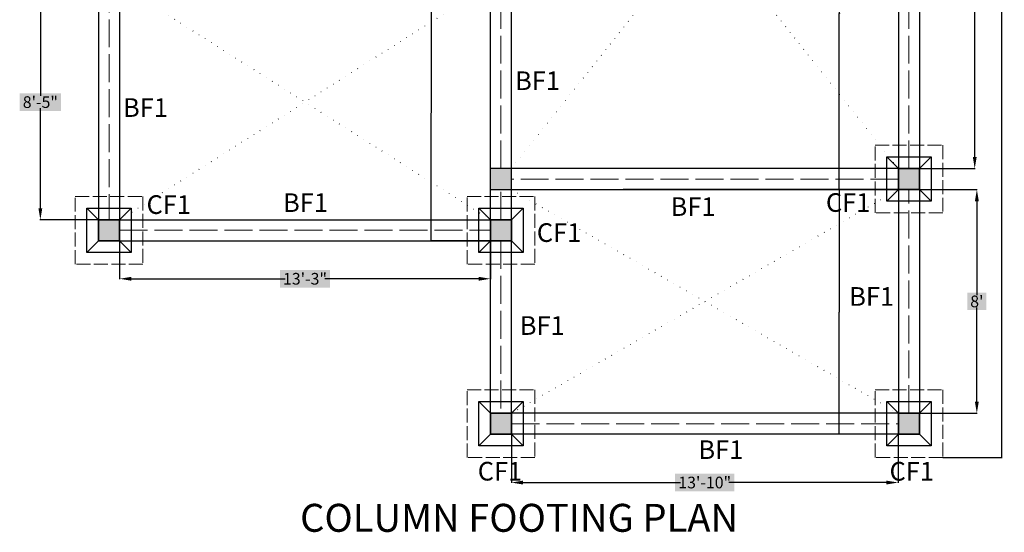
# Model space of a CAD drawing. Units: inches. Extents: x -35 to 832, y -515 to 219.
# Tile 6 of 7: x 410 to 832, y -295 to -75. Entities that reach past the tile are written whole.
import ezdxf

# ---------------------------------------------------------------- set-up
doc = ezdxf.new("R2010")
doc.units = ezdxf.units.IN
doc.header["$MEASUREMENT"] = 0
doc.linetypes.add('ACAD_ISO02W100', pattern=[15, 12, -3])
doc.linetypes.add('ACAD_ISO07W100', pattern=[3, 0, -3])
for name, color, linetype, lineweight in [('G-ANNO-TEXT', 7, 'Continuous', 35), ('S-ANNO-DIMS', 2, 'Continuous', 18), ('S-ANNO-TEXT', 7, 'Continuous', 18), ('S-BEAM', 6, 'Continuous', 25), ('S-BEAM-CNTR', 2, 'ACAD_ISO02W100', 13), ('S-COLS', 4, 'Continuous', 35), ('S-COLS-PATT', 8, 'Continuous', 13), ('S-FNDN', 4, 'Continuous', 25), ('S-FNDN-HIDN', 7, 'ACAD_ISO02W100', 18), ('S-FNDN-REFR', 8, 'ACAD_ISO07W100', 13)]:
    doc.layers.add(name, color=color, linetype=linetype, lineweight=lineweight)
doc.styles.get("Standard").update_dxf_attribs({"font": 'arial.ttf'})
doc.dimstyles.get("Standard").update_dxf_attribs({"dimtxt": 0.18, "dimasz": 0.18, "dimexe": 0.18, "dimexo": 0.0625, "dimgap": 0.09, "dimtad": 0, "dimtih": 1, "dimtoh": 1, "dimdec": 1, "dimzin": 0, "dimdsep": 46, "dimlunit": 4, "dimtxsty": 'Standard', "dimcen": 0.09, "dimclrd": 211, "dimclre": 4, "dimclrt": 3, "dimadec": 0, "dimazin": 0, "dimtfac": 0.5, "dimtdec": 1, "dimtofl": 0, "dimtmove": 0, "dimatfit": 3, "dimfxl": 1, "dimtfill": 2, "dimtfillclr": 61, "dimtolj": 1, "dimtzin": 0, "dimarcsym": 0})

# ---------------------------------------------------------------- blocks, each defined once
blk = doc.blocks.new('*D28')
at = {"layer": 'Defpoints', "color": 0, "transparency": 16777216}
for p in [(620.57, -248.58), (786.4, -248.58), (786.4, -273.78)]:
    blk.add_point(p, dxfattribs=at)
at = {"layer": 'S-ANNO-DIMS', "color": 0, "lineweight": -2, "transparency": 16777216}
for p, q in [((620.57, -248.64), (620.57, -273.96)), ((786.4, -248.64), (786.4, -273.96)), ((625.57, -273.78), (693.1, -273.78)), ((781.4, -273.78), (713.87, -273.78))]:
    blk.add_line(p, q, dxfattribs=at)
at = {"layer": 'S-ANNO-DIMS', "color": 0, "transparency": 16777216}
for points in [[(625.57, -272.95), (625.57, -274.62), (620.57, -273.78)], [(781.4, -272.95), (781.4, -274.62), (786.4, -273.78)]]:
    blk.add_solid(points, dxfattribs=at)
at = {"layer": 'S-ANNO-DIMS', "color": 0, "transparency": 16777216, "insert": (703.49, -273.78), "char_height": 5, "attachment_point": 5, "bg_fill": 1, "box_fill_scale": 1.25, "bg_fill_color": 61, "bg_fill_transparency": 0}
blk.add_mtext('\\A1;13\'-10"', dxfattribs=at)
blk = doc.blocks.new('*D29')
at = {"layer": 'Defpoints', "color": 0, "transparency": 16777216}
for p in [(452.57, -165.58), (611.57, -165.58), (611.57, -186.37)]:
    blk.add_point(p, dxfattribs=at)
at = {"layer": 'S-ANNO-DIMS', "color": 0, "lineweight": -2, "transparency": 16777216}
for p, q in [((452.57, -165.64), (452.57, -186.55)), ((611.57, -165.64), (611.57, -186.55)), ((457.57, -186.37), (523.63, -186.37)), ((606.57, -186.37), (540.51, -186.37))]:
    blk.add_line(p, q, dxfattribs=at)
at = {"layer": 'S-ANNO-DIMS', "color": 0, "transparency": 16777216}
for points in [[(457.57, -185.54), (457.57, -187.21), (452.57, -186.37)], [(606.57, -185.54), (606.57, -187.21), (611.57, -186.37)]]:
    blk.add_solid(points, dxfattribs=at)
at = {"layer": 'S-ANNO-DIMS', "color": 0, "transparency": 16777216, "insert": (532.07, -186.37), "char_height": 5, "attachment_point": 5, "bg_fill": 1, "box_fill_scale": 1.25, "bg_fill_color": 61, "bg_fill_transparency": 0}
blk.add_mtext('\\A1;13\'-3"', dxfattribs=at)
blk = doc.blocks.new('*D30')
at = {"layer": 'Defpoints', "color": 0, "transparency": 16777216}
for p in [(786.57, -148.08), (786.57, -244.08), (820.2, -244.08)]:
    blk.add_point(p, dxfattribs=at)
at = {"layer": 'S-ANNO-DIMS', "color": 0, "lineweight": -2, "transparency": 16777216}
for p, q in [((786.63, -148.08), (820.38, -148.08)), ((820.2, -153.08), (820.2, -193.43)), ((820.2, -239.08), (820.2, -198.72)), ((786.63, -244.08), (820.38, -244.08))]:
    blk.add_line(p, q, dxfattribs=at)
at = {"layer": 'S-ANNO-DIMS', "color": 0, "transparency": 16777216}
for points in [[(819.37, -153.08), (821.03, -153.08), (820.2, -148.08)], [(819.37, -239.08), (821.03, -239.08), (820.2, -244.08)]]:
    blk.add_solid(points, dxfattribs=at)
at = {"layer": 'S-ANNO-DIMS', "color": 0, "transparency": 16777216, "insert": (820.2, -196.08), "char_height": 5, "attachment_point": 5, "bg_fill": 1, "box_fill_scale": 1.25, "bg_fill_color": 61, "bg_fill_transparency": 0}
blk.add_mtext("\\A1;8'", dxfattribs=at)
blk = doc.blocks.new('*D31')
at = {"layer": 'Defpoints', "color": 0, "transparency": 16777216}
for p in [(786.57, 2.92), (819.29, 2.92), (786.57, -139.08)]:
    blk.add_point(p, dxfattribs=at)
at = {"layer": 'S-ANNO-DIMS', "color": 0, "lineweight": -2, "transparency": 16777216}
for p, q in [((786.63, 2.92), (819.47, 2.92)), ((819.29, -2.08), (819.29, -65.43)), ((819.29, -134.08), (819.29, -70.72)), ((786.63, -139.08), (819.47, -139.08))]:
    blk.add_line(p, q, dxfattribs=at)
at = {"layer": 'S-ANNO-DIMS', "color": 0, "transparency": 16777216}
for points in [[(818.46, -2.08), (820.13, -2.08), (819.29, 2.92)], [(818.46, -134.08), (820.13, -134.08), (819.29, -139.08)]]:
    blk.add_solid(points, dxfattribs=at)
at = {"layer": 'S-ANNO-DIMS', "color": 0, "transparency": 16777216, "insert": (819.29, -68.08), "char_height": 5, "attachment_point": 5, "bg_fill": 1, "box_fill_scale": 1.25, "bg_fill_color": 61, "bg_fill_transparency": 0}
blk.add_mtext('\\A1;11\'-10"', dxfattribs=at)
blk = doc.blocks.new('*D38')
at = {"layer": 'Defpoints', "color": 0, "transparency": 16777216}
for p in [(448.07, -60.08), (418.57, -161.08), (448.07, -161.08)]:
    blk.add_point(p, dxfattribs=at)
at = {"layer": 'S-ANNO-DIMS', "color": 0, "lineweight": -2, "transparency": 16777216}
for p, q in [((448.01, -60.08), (418.39, -60.08)), ((418.57, -65.08), (418.57, -107.93)), ((418.57, -156.08), (418.57, -113.22)), ((448.01, -161.08), (418.39, -161.08))]:
    blk.add_line(p, q, dxfattribs=at)
at = {"layer": 'S-ANNO-DIMS', "color": 0, "transparency": 16777216}
for points in [[(417.74, -65.08), (419.41, -65.08), (418.57, -60.08)], [(417.74, -156.08), (419.41, -156.08), (418.57, -161.08)]]:
    blk.add_solid(points, dxfattribs=at)
at = {"layer": 'S-ANNO-DIMS', "color": 0, "transparency": 16777216, "insert": (418.57, -110.58), "char_height": 5, "attachment_point": 5, "bg_fill": 1, "box_fill_scale": 1.25, "bg_fill_color": 61, "bg_fill_transparency": 0}
blk.add_mtext('\\A1;8\'-5"', dxfattribs=at)
blk = doc.blocks.new('CF1-TAPERED-FOOTING')
for p, q in [((0, 19), (19, 19)), ((0, 0), (0, 19)), ((0, 19), (5, 14)), ((14, 14), (19, 19)), ((19, 19), (19, 0)), ((0, 0), (5, 5)), ((14, 5), (19, 0)), ((19, 0), (0, 0))]:
    blk.add_line(p, q)
blk = doc.blocks.new('CF1-FOOTING-LIMIT')
at = {"ltscale": 0.5}
for p, q in [((0, 29), (29, 29)), ((0, 0), (0, 29)), ((29, 29), (29, 0)), ((29, 0), (0, 0))]:
    blk.add_line(p, q, dxfattribs=at)
blk = doc.blocks.new('*D140')
at = {"layer": 'Defpoints', "color": 0, "transparency": 16777216}
for p in [(805.57, 193.92), (805.57, -263.08), (830.92, -263.08)]:
    blk.add_point(p, dxfattribs=at)
at = {"layer": 'S-ANNO-DIMS', "color": 4, "lineweight": -2, "transparency": 16777216}
for p, q in [((805.63, 193.92), (831.1, 193.92)), ((805.63, -263.08), (831.1, -263.08))]:
    blk.add_line(p, q, dxfattribs=at)
at = {"layer": 'S-ANNO-DIMS', "color": 211, "lineweight": -2, "transparency": 16777216}
for p, q in [((830.92, 193.74), (830.92, -34.39)), ((830.92, -262.9), (830.92, -34.76))]:
    blk.add_line(p, q, dxfattribs=at)
at = {"layer": 'S-ANNO-DIMS', "color": 211, "transparency": 16777216}
for points in [[(830.89, 193.74), (830.95, 193.74), (830.92, 193.92)], [(830.89, -262.9), (830.95, -262.9), (830.92, -263.08)]]:
    blk.add_solid(points, dxfattribs=at)
at = {"layer": 'S-ANNO-DIMS', "color": 3, "transparency": 16777216, "insert": (830.92, -34.58), "char_height": 0.18, "attachment_point": 5, "bg_fill": 1, "box_fill_scale": 1.25, "bg_fill_color": 61, "bg_fill_transparency": 0}
blk.add_mtext('\\A1;38\'-1"', dxfattribs=at)
blk = doc.blocks.new('*D145')
at = {"layer": 'Defpoints', "color": 0, "transparency": 16777216}
for p in [(586.22, -60.08), (611.57, -60.08), (611.57, -170.08)]:
    blk.add_point(p, dxfattribs=at)
at = {"layer": 'S-ANNO-DIMS', "color": 4, "lineweight": -2, "transparency": 16777216}
for p, q in [((611.51, -60.08), (586.04, -60.08)), ((611.51, -170.08), (586.04, -170.08))]:
    blk.add_line(p, q, dxfattribs=at)
at = {"layer": 'S-ANNO-DIMS', "color": 211, "lineweight": -2, "transparency": 16777216}
for p, q in [((586.22, -60.26), (586.22, -114.89)), ((586.22, -169.9), (586.22, -115.26))]:
    blk.add_line(p, q, dxfattribs=at)
at = {"layer": 'S-ANNO-DIMS', "color": 211, "transparency": 16777216}
for points in [[(586.19, -60.26), (586.25, -60.26), (586.22, -60.08)], [(586.19, -169.9), (586.25, -169.9), (586.22, -170.08)]]:
    blk.add_solid(points, dxfattribs=at)
at = {"layer": 'S-ANNO-DIMS', "color": 3, "transparency": 16777216, "insert": (586.22, -115.08), "char_height": 0.18, "attachment_point": 5, "bg_fill": 1, "box_fill_scale": 1.25, "bg_fill_color": 61, "bg_fill_transparency": 0}
blk.add_mtext('\\A1;9\'-2"', dxfattribs=at)
blk = doc.blocks.new('*D148')
at = {"layer": 'Defpoints', "color": 0, "transparency": 16777216}
for p in [(761.22, 2.92), (786.57, 2.92), (786.57, -148.08)]:
    blk.add_point(p, dxfattribs=at)
at = {"layer": 'S-ANNO-DIMS', "color": 4, "lineweight": -2, "transparency": 16777216}
for p, q in [((786.51, 2.92), (761.04, 2.92)), ((786.51, -148.08), (761.04, -148.08))]:
    blk.add_line(p, q, dxfattribs=at)
at = {"layer": 'S-ANNO-DIMS', "color": 211, "lineweight": -2, "transparency": 16777216}
for p, q in [((761.22, 2.74), (761.22, -72.39)), ((761.22, -147.9), (761.22, -72.76))]:
    blk.add_line(p, q, dxfattribs=at)
at = {"layer": 'S-ANNO-DIMS', "color": 211, "transparency": 16777216}
for points in [[(761.19, 2.74), (761.25, 2.74), (761.22, 2.92)], [(761.19, -147.9), (761.25, -147.9), (761.22, -148.08)]]:
    blk.add_solid(points, dxfattribs=at)
at = {"layer": 'S-ANNO-DIMS', "color": 3, "transparency": 16777216, "insert": (761.22, -72.58), "char_height": 0.18, "attachment_point": 5, "bg_fill": 1, "box_fill_scale": 1.25, "bg_fill_color": 61, "bg_fill_transparency": 0}
blk.add_mtext('\\A1;12\'-7"', dxfattribs=at)
blk = doc.blocks.new('*D149')
at = {"layer": 'Defpoints', "color": 0, "transparency": 16777216}
for p in [(761.22, -148.08), (786.57, -148.08), (786.57, -253.08)]:
    blk.add_point(p, dxfattribs=at)
at = {"layer": 'S-ANNO-DIMS', "color": 4, "lineweight": -2, "transparency": 16777216}
for p, q in [((786.51, -148.08), (761.04, -148.08)), ((786.51, -253.08), (761.04, -253.08))]:
    blk.add_line(p, q, dxfattribs=at)
at = {"layer": 'S-ANNO-DIMS', "color": 211, "lineweight": -2, "transparency": 16777216}
for p, q in [((761.22, -148.26), (761.22, -200.39)), ((761.22, -252.9), (761.22, -200.76))]:
    blk.add_line(p, q, dxfattribs=at)
at = {"layer": 'S-ANNO-DIMS', "color": 211, "transparency": 16777216}
for points in [[(761.19, -148.26), (761.25, -148.26), (761.22, -148.08)], [(761.19, -252.9), (761.25, -252.9), (761.22, -253.08)]]:
    blk.add_solid(points, dxfattribs=at)
at = {"layer": 'S-ANNO-DIMS', "color": 3, "transparency": 16777216, "insert": (761.22, -200.58), "char_height": 0.18, "attachment_point": 5, "bg_fill": 1, "box_fill_scale": 1.25, "bg_fill_color": 61, "bg_fill_transparency": 0}
blk.add_mtext('\\A1;8\'-9"', dxfattribs=at)

msp = doc.modelspace()

# ---------------------------------------------------------------- hatches: boundary and pattern name
at = {"layer": 'S-COLS-PATT'}
h = msp.add_hatch(color=256, dxfattribs=at)
h.dxf.hatch_style = 1
h.paths.add_polyline_path([(443.57, 183.92), (443.57, 174.92), (452.57, 174.92), (452.57, 183.92)])
h.paths.add_polyline_path([(620.57, 183.92), (611.57, 183.92), (611.57, 174.92), (620.57, 174.92)])
h.paths.add_polyline_path([(786.57, 183.92), (786.57, 174.92), (795.57, 174.92), (795.57, 183.92)])
h.paths.add_polyline_path([(620.57, 78.92), (611.57, 78.92), (611.57, 69.92), (620.57, 69.92)])
h.paths.add_polyline_path([(659.57, 78.92), (659.57, 69.92), (668.57, 69.92), (668.57, 78.92)])
h.paths.add_polyline_path([(795.57, 78.92), (786.57, 78.92), (786.57, 69.92), (795.57, 69.92)])
h.paths.add_polyline_path([(668.57, 11.92), (659.57, 11.92), (659.57, 2.92), (668.57, 2.92)])
h.paths.add_polyline_path([(795.57, 11.92), (786.57, 11.92), (786.57, 2.92), (795.57, 2.92)])
h.paths.add_polyline_path([(611.57, 17.92), (611.57, 8.92), (620.57, 8.92), (620.57, 17.92)])
h.paths.add_polyline_path([(557.57, 17.92), (548.57, 17.92), (548.57, 8.92), (557.57, 8.92)])
h.paths.add_polyline_path([(443.57, 8.92), (452.57, 8.92), (452.57, 17.92), (443.57, 17.92)])
h.paths.add_polyline_path([(443.57, -51.08), (443.57, -60.08), (452.57, -60.08), (452.57, -51.08)])
h.paths.add_polyline_path([(557.57, -51.08), (548.57, -51.08), (548.57, -60.08), (557.57, -60.08)])
h.paths.add_polyline_path([(620.57, -60.08), (620.57, -51.08), (611.57, -51.08), (611.57, -60.08)])
h.paths.add_polyline_path([(620.57, -139.08), (611.57, -139.08), (611.57, -148.08), (620.57, -148.08)])
h.paths.add_polyline_path([(786.57, -148.08), (795.57, -148.08), (795.57, -139.08), (786.57, -139.08)])
h.paths.add_polyline_path([(443.57, -161.08), (443.57, -170.08), (452.57, -170.08), (452.57, -161.08)])
h.paths.add_polyline_path([(611.57, -161.08), (611.57, -170.08), (620.57, -170.08), (620.57, -161.08)])
h.paths.add_polyline_path([(620.57, -244.08), (611.57, -244.08), (611.57, -253.08), (620.57, -253.08)])
h.paths.add_polyline_path([(786.57, -244.08), (786.57, -253.08), (795.57, -253.08), (795.57, -244.08)])

# ---------------------------------------------------------------- linework, layer by layer
at = {"layer": 'S-BEAM'}
for p, q in [((611.57, -142.58), (611.57, 78.92)), ((620.57, -142.58), (620.57, 69.92)), ((795.57, 11.92), (795.57, -139.08)), ((786.57, 2.92), (786.57, -139.08)), ((443.57, -51.08), (443.57, -170.08)), ((452.57, -60.08), (452.57, -161.08)), ((795.57, -60.08), (795.57, -253.08)), ((786.57, -139.08), (611.57, -139.08)), ((611.57, -253.08), (611.57, -139.08)), ((620.57, -244.08), (620.57, -139.08)), ((611.57, -148.08), (786.57, -148.08)), ((786.57, -148.08), (668.57, -148.08)), ((786.57, -148.08), (786.57, -244.08)), ((452.57, -161.08), (620.57, -161.08)), ((443.57, -170.08), (611.57, -170.08)), ((786.57, -244.08), (620.57, -244.08)), ((795.57, -253.08), (611.57, -253.08))]:
    msp.add_line(p, q, dxfattribs=at)
at = {"layer": 'S-BEAM-CNTR'}
for p, q in [((616.07, -139.08), (616.07, 74.42)), ((791.07, -139.08), (791.07, 2.92)), ((448.07, -60.08), (448.07, -161.08)), ((786.57, -143.58), (620.57, -143.58)), ((616.07, -161.08), (616.07, -148.08)), ((791.07, -244.08), (791.07, -148.08)), ((452.57, -165.58), (611.57, -165.58)), ((616.07, -170.08), (616.07, -244.08)), ((620.57, -248.58), (786.57, -248.58))]:
    msp.add_line(p, q, dxfattribs=at)
at = {"layer": 'S-COLS'}
for p, q in [((786.57, -139.08), (795.57, -139.08)), ((786.57, -148.08), (786.57, -139.08)), ((795.57, -139.08), (795.57, -148.08)), ((795.57, -148.08), (786.57, -148.08)), ((443.57, -161.08), (452.57, -161.08)), ((443.57, -170.08), (443.57, -161.08)), ((452.57, -161.08), (452.57, -170.08)), ((611.57, -161.08), (620.57, -161.08)), ((611.57, -170.08), (611.57, -161.08)), ((620.57, -161.08), (620.57, -170.08)), ((452.57, -170.08), (443.57, -170.08)), ((620.57, -170.08), (611.57, -170.08)), ((611.57, -244.08), (620.57, -244.08)), ((611.57, -253.08), (611.57, -244.08)), ((620.57, -244.08), (620.57, -253.08)), ((786.57, -244.08), (795.57, -244.08)), ((786.57, -253.08), (786.57, -244.08)), ((795.57, -244.08), (795.57, -253.08)), ((620.57, -253.08), (611.57, -253.08)), ((795.57, -253.08), (786.57, -253.08))]:
    msp.add_line(p, q, dxfattribs=at)
at = {"layer": 'S-FNDN-REFR'}
for p, q in [((620.57, 69.92), (786.57, -139.08)), ((620.57, -139.08), (786.57, 69.92)), ((452.57, -60.08), (611.57, -161.08)), ((452.57, -161.08), (611.57, -60.08)), ((620.39, -148.08), (786.57, -244.08)), ((620.57, -244.08), (786.57, -148.08))]:
    msp.add_line(p, q, dxfattribs=at)

# ---------------------------------------------------------------- block references
at = {"layer": 'S-FNDN'}
for p in [(781.57, -153.07), (438.57, -175.07), (606.57, -258.07), (781.57, -258.07)]:
    msp.add_blockref('CF1-TAPERED-FOOTING', p, dxfattribs=at)
at = {"layer": 'S-FNDN', "rotation": 180}
msp.add_blockref('CF1-TAPERED-FOOTING', (625.57, -156.08), dxfattribs=at)
at = {"layer": 'S-FNDN-HIDN'}
for p, rotation in [((805.57, -158.08), 90.00000000000028), ((462.57, -180.08), 89.99999999999991), ((601.57, -151.07), 270.0000000000001), ((630.57, -263.08), 90.0000000000001), ((805.57, -263.08), 90.00000000000017)]:
    msp.add_blockref('CF1-FOOTING-LIMIT', p, dxfattribs=dict(at, rotation=rotation))

# ---------------------------------------------------------------- texts
at = {"layer": 'G-ANNO-TEXT', "insert": (529.97, -282.92), "char_height": 12, "attachment_point": 1}
msp.add_mtext_dynamic_manual_height_columns('COLUMN FOOTING PLAN', width=219.0757, gutter_width=1, heights=[0], dxfattribs=at)
at = {"layer": 'S-ANNO-TEXT'}
for s, p in [('BF1', (622.17, -105.41)), ('BF1', (454.02, -116.92)), ('CF1', (464.12, -158.56)), ('BF1', (522.66, -157.72)), ('BF1', (688.87, -159.42)), ('CF1', (755.47, -157.66)), ('CF1', (631.5, -170.56)), ('BF1', (765.46, -197.95)), ('BF1', (624.2, -210.42)), ('BF1', (700.79, -263.69)), ('CF1', (606.15, -272.92)), ('CF1', (782.76, -272.96))]:
    msp.add_text(s, height=8, dxfattribs=at).set_placement(p)

# ---------------------------------------------------------------- dimensions: what is measured, and where the dimension line sits
at = {"layer": 'S-ANNO-DIMS'}
for base, p1, p2, override, picture, middle in [((830.92, -263.08), (805.57, 193.92), (805.57, -263.08), {"dimdec": 1, "dimlfac": 1, "dimrnd": 0, "dimzin": 1, "dimdsep": 46, "dimlunit": 4, "dimfrac": 2}, '*D140', (830.92, -34.58)), ((761.22, 2.92), (786.57, -148.08), (786.57, 2.92), {"dimdec": 1, "dimlfac": 1, "dimrnd": 0, "dimzin": 1, "dimdsep": 46, "dimlunit": 4, "dimfrac": 2}, '*D148', (761.22, -72.58)), ((819.29, 2.92), (786.57, -139.08), (786.57, 2.92), {"dimtxt": 5, "dimasz": 5, "dimclrd": 0, "dimclre": 0, "dimclrt": 0}, '*D31', (819.29, -68.08)), ((418.57, -161.08), (448.07, -60.08), (448.07, -161.08), {"dimtxt": 5, "dimasz": 5, "dimclrd": 0, "dimclre": 0, "dimclrt": 0}, '*D38', (418.57, -110.58)), ((586.22, -60.08), (611.57, -170.08), (611.57, -60.08), {"dimdec": 1, "dimlfac": 1, "dimrnd": 0, "dimzin": 1, "dimdsep": 46, "dimlunit": 4, "dimfrac": 2}, '*D145', (586.22, -115.08)), ((761.22, -148.08), (786.57, -253.08), (786.57, -148.08), {"dimdec": 1, "dimlfac": 1, "dimrnd": 0, "dimzin": 1, "dimdsep": 46, "dimlunit": 4, "dimfrac": 2}, '*D149', (761.22, -200.58)), ((820.2, -244.08), (786.57, -148.08), (786.57, -244.08), {"dimtxt": 5, "dimasz": 5, "dimclrd": 0, "dimclre": 0, "dimclrt": 0}, '*D30', (820.2, -196.08))]:
    dim = msp.add_linear_dim(base=base, p1=p1, p2=p2, angle=90, dimstyle='Standard', override=override, dxfattribs=at)
    dim.commit()
    dim.dimension.update_dxf_attribs({"geometry": picture, "text_midpoint": middle})
for base, p1, p2, picture, middle in [((611.57, -186.37), (452.57, -165.58), (611.57, -165.58), '*D29', (532.07, -186.37)), ((786.4, -273.78), (620.57, -248.58), (786.4, -248.58), '*D28', (703.49, -273.78))]:
    dim = msp.add_linear_dim(base=base, p1=p1, p2=p2, dimstyle='Standard', override={"dimtxt": 5, "dimasz": 5, "dimclrd": 0, "dimclre": 0, "dimclrt": 0}, dxfattribs=at)
    dim.commit()
    dim.dimension.update_dxf_attribs({"geometry": picture, "text_midpoint": middle})

doc.saveas('drawing.dxf')
